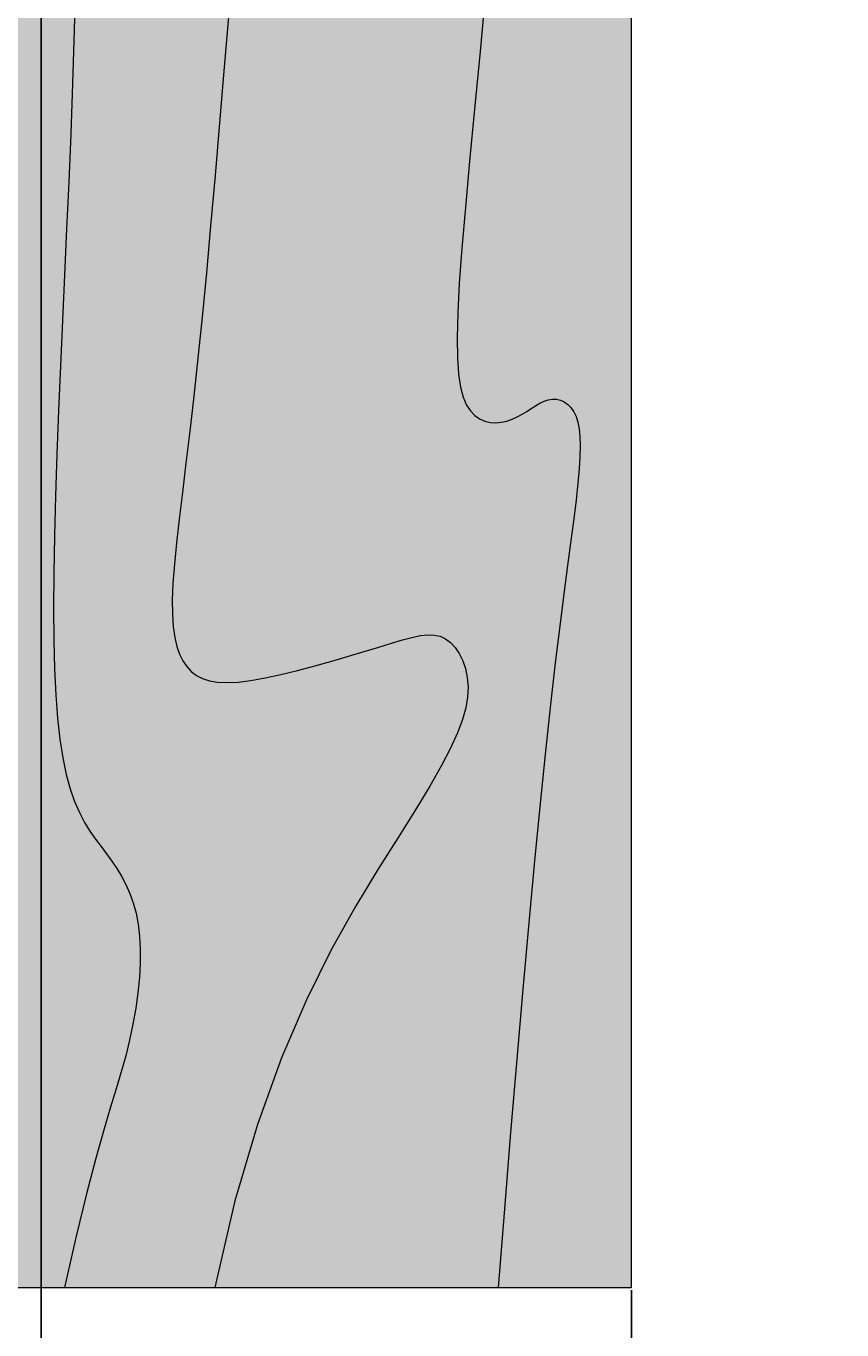
# Model space of a CAD drawing. Units: inches. Extents: x 2549 to 3108, y 1683 to 2362.
# Tile 25 of 30: x 2966 to 2985, y 2018 to 2049. Entities that reach past the tile are written whole.
import ezdxf

# ---------------------------------------------------------------- set-up
doc = ezdxf.new("R2010")
doc.units = ezdxf.units.IN
for name, color, linetype, lineweight in [('A-ANNO-DIMS', 2, 'Continuous', 18), ('A-FURN', 8, 'Continuous', 18), ('A-FURN-PATT', 9, 'Continuous', 13)]:
    doc.layers.add(name, color=color, linetype=linetype, lineweight=lineweight)
doc.layers.add('C-PKNG-VEHI-PATT', color=251, linetype='Continuous', lineweight=13, true_color=0x636466)
doc.layers.add('C-PVMT-PATT', color=9, linetype='Continuous', lineweight=13, true_color=0xc7c8ca)
doc.styles.get("Standard").update_dxf_attribs({"font": 'arial.ttf'})
doc.dimstyles.get("Standard").update_dxf_attribs({"dimtxt": 0.18, "dimasz": 0.18, "dimexe": 0.18, "dimexo": 0.0625, "dimgap": 0.09, "dimtad": 0, "dimtih": 1, "dimtoh": 1, "dimdec": 4, "dimzin": 0, "dimdsep": 46, "dimtxsty": 'Standard', "dimcen": 0.09, "dimadec": 0, "dimazin": 0, "dimtfac": 1, "dimtdec": 4, "dimtofl": 0, "dimtmove": 0, "dimatfit": 3, "dimfxl": 1, "dimtolj": 1, "dimtzin": 0, "dimarcsym": 0})

# ---------------------------------------------------------------- blocks, each defined once
blk = doc.blocks.new('Table - Rectangular Woodgrain 60 x 30 in.')
for p, q in [((60, 0), (0, 0)), ((60, -30), (60, 0))]:
    blk.add_line(p, q)
for points in [[(28.8172, -3.4958), (30.3437, -3.636), (31.7291, -3.7667), (32.9756, -3.8849), (34.0849, -3.9875), (35.059, -4.0714), (35.9, -4.1334), (36.6114, -4.1711), (37.2041, -4.1854), (37.6906, -4.1779), (38.0833, -4.15), (38.3948, -4.1034), (38.6375, -4.0396), (38.8239, -3.9602), (38.9666, -3.8667), (39.0764, -3.7608), (39.1573, -3.6448), (39.2116, -3.521), (39.2416, -3.3917), (39.2498, -3.2593), (39.2385, -3.1261), (39.21, -2.9944), (39.1666, -2.8667), (39.111, -2.7447), (39.0468, -2.6281), (38.978, -2.5163), (38.9083, -2.4083), (38.8418, -2.3035), (38.7823, -2.201), (38.7337, -2.1001), (38.7, -2), (38.6844, -1.9003), (38.6875, -1.8021), (38.7094, -1.707), (38.75, -1.6167), (38.8094, -1.5326), (38.8875, -1.4563), (38.9844, -1.3893), (39.1, -1.3333), (39.2351, -1.2896), (39.3937, -1.2583), (39.5804, -1.2396), (39.8, -1.2333), (40.057, -1.2396), (40.3562, -1.2583), (40.7023, -1.2896), (41.1, -1.3333), (41.5547, -1.3895), (42.0755, -1.4573), (42.6721, -1.5361), (43.3542, -1.625), (44.1316, -1.7233), (45.014, -1.8302), (46.0114, -1.9449), (47.1333, -2.0667), (48.3862, -2.1947), (49.7625, -2.3281), (51.2513, -2.4663), (52.8416, -2.6083), (54.5226, -2.7535), (56.2833, -2.9011), (58.1127, -3.0501), (60, -3.2)], [(29.3241, -9.6553), (30.7203, -9.7719), (32.0532, -9.8837), (33.3208, -9.9917), (34.5213, -10.0965), (35.6526, -10.199), (36.7128, -10.2999), (37.7, -10.4), (38.6129, -10.4996), (39.4531, -10.5969), (40.223, -10.6895), (40.925, -10.775), (41.5613, -10.8512), (42.1344, -10.9156), (42.6465, -10.966), (43.1, -11), (43.4976, -11.0158), (43.8437, -11.0136), (44.143, -10.9942), (44.4, -10.9583), (44.6195, -10.9069), (44.8062, -10.8406), (44.9648, -10.7603), (45.1, -10.6667), (45.2155, -10.5598), (45.3114, -10.4365), (45.3871, -10.2929), (45.4416, -10.125), (45.4743, -9.929), (45.4844, -9.7011), (45.4709, -9.4371), (45.4333, -9.1333), (45.3716, -8.7883), (45.2896, -8.4104), (45.1919, -8.0107), (45.0833, -7.6), (44.9685, -7.1893), (44.8521, -6.7896), (44.7388, -6.4117), (44.6333, -6.0667), (44.54, -5.7628), (44.4614, -5.4979), (44.4001, -5.2675), (44.3583, -5.0667), (44.3384, -4.8909), (44.3427, -4.7354), (44.3736, -4.5956), (44.4333, -4.4667), (44.5236, -4.3453), (44.6427, -4.2333), (44.7884, -4.1339), (44.9583, -4.05), (45.1501, -3.9849), (45.3614, -3.9417), (45.59, -3.9234), (45.8333, -3.9333), (46.0915, -3.9749), (46.3734, -4.0531), (46.6906, -4.1736), (47.0542, -4.3417), (47.4756, -4.5629), (47.9661, -4.8427), (48.5372, -5.1866), (49.2, -5.6), (49.9676, -6.0844), (50.8594, -6.625), (51.8965, -7.2031), (53.1, -7.8), (54.491, -8.3969), (56.0906, -8.975), (57.9199, -9.5156), (60, -10)], [(28.4531, -13.3281), (29.8256, -13.3663), (31.1083, -13.4083), (32.3191, -13.4535), (33.476, -13.501), (34.597, -13.5501), (35.7, -13.6), (36.7984, -13.6497), (37.8875, -13.6979), (38.9578, -13.743), (40, -13.7833), (41.0047, -13.8174), (41.9625, -13.8438), (42.864, -13.8607), (43.7, -13.8667), (44.4631, -13.8604), (45.1552, -13.8417), (45.7801, -13.8104), (46.3416, -13.7667), (46.8439, -13.7104), (47.2906, -13.6417), (47.6858, -13.5604), (48.0333, -13.4667), (48.3375, -13.3608), (48.6042, -13.2448), (48.8396, -13.121), (49.05, -12.9917), (49.2417, -12.8593), (49.4208, -12.7261), (49.5937, -12.5944), (49.7667, -12.4667), (49.9452, -12.3451), (50.1323, -12.2313), (50.3303, -12.1268), (50.5416, -12.0333), (50.7686, -11.9524), (51.0135, -11.8854), (51.2788, -11.8341), (51.5666, -11.8), (51.8785, -11.7843), (52.2116, -11.7865), (52.562, -11.8059), (52.926, -11.8417), (53.2998, -11.8931), (53.6795, -11.9594), (54.0614, -12.0397), (54.4416, -12.1333), (54.8223, -12.2401), (55.2293, -12.3625), (55.6942, -12.5037), (56.2489, -12.6667), (56.9251, -12.8547), (57.7545, -13.0708), (58.7689, -13.3182), (60, -13.6)]]:
    blk.add_lwpolyline(points)
blk = doc.blocks.new('*D23')
at = {"layer": 'A-ANNO-DIMS', "color": 0, "lineweight": -2, "transparency": 16777216}
for p, q in [((2950.093, 2018.552), (2950.093, 2009.435)), ((2980.093, 2018.552), (2980.093, 2009.435)), ((2950.273, 2009.615), (2964.875, 2009.615)), ((2979.913, 2009.615), (2965.312, 2009.615))]:
    blk.add_line(p, q, dxfattribs=at)
at = {"layer": 'A-ANNO-DIMS', "color": 0, "transparency": 16777216}
for points in [[(2950.273, 2009.645), (2950.273, 2009.585), (2950.093, 2009.615)], [(2979.913, 2009.645), (2979.913, 2009.585), (2980.093, 2009.615)]]:
    blk.add_solid(points, dxfattribs=at)
at = {"layer": 'Defpoints', "color": 0, "transparency": 16777216}
for p in [(2950.093, 2018.615), (2980.093, 2018.615), (2980.093, 2009.615)]:
    blk.add_point(p, dxfattribs=at)
at = {"layer": 'A-ANNO-DIMS', "color": 0, "transparency": 16777216, "insert": (2965.093, 2009.615), "char_height": 0.18, "attachment_point": 5}
blk.add_mtext('\\A1;30', dxfattribs=at)
blk = doc.blocks.new('*D46')
at = {"layer": 'A-ANNO-DIMS', "color": 0, "lineweight": -2, "transparency": 16777216}
for p, q in [((2812.643, 2140.461), (2812.643, 1683.444)), ((3034.643, 2134.461), (3034.643, 1683.444)), ((2812.823, 1683.624), (2923.353, 1683.624)), ((3034.463, 1683.624), (2923.932, 1683.624))]:
    blk.add_line(p, q, dxfattribs=at)
at = {"layer": 'A-ANNO-DIMS', "color": 0, "transparency": 16777216}
for points in [[(2812.823, 1683.654), (2812.823, 1683.594), (2812.643, 1683.624)], [(3034.463, 1683.654), (3034.463, 1683.594), (3034.643, 1683.624)]]:
    blk.add_solid(points, dxfattribs=at)
at = {"layer": 'Defpoints', "color": 0, "transparency": 16777216}
for p in [(2812.643, 2140.524), (3034.643, 2134.524), (3034.643, 1683.624)]:
    blk.add_point(p, dxfattribs=at)
at = {"layer": 'A-ANNO-DIMS', "color": 0, "transparency": 16777216, "insert": (2923.643, 1683.624), "char_height": 0.18, "attachment_point": 5}
blk.add_mtext('\\A1;222', dxfattribs=at)
blk = doc.blocks.new('*D57')
at = {"layer": 'A-ANNO-DIMS', "color": 0, "lineweight": -2, "transparency": 16777216}
for p, q in [((2965.935, 1936.586), (2965.935, 2362.323)), ((3034.643, 1936.586), (3034.643, 2362.323)), ((2966.115, 2362.143), (2999.912, 2362.143)), ((3034.463, 2362.143), (3000.666, 2362.143))]:
    blk.add_line(p, q, dxfattribs=at)
at = {"layer": 'A-ANNO-DIMS', "color": 0, "transparency": 16777216}
for points in [[(2966.115, 2362.173), (2966.115, 2362.113), (2965.935, 2362.143)], [(3034.463, 2362.173), (3034.463, 2362.113), (3034.643, 2362.143)]]:
    blk.add_solid(points, dxfattribs=at)
at = {"layer": 'Defpoints', "color": 0, "transparency": 16777216}
for p in [(3034.643, 2362.143), (2965.935, 1936.524), (3034.643, 1936.524)]:
    blk.add_point(p, dxfattribs=at)
at = {"layer": 'A-ANNO-DIMS', "color": 0, "transparency": 16777216, "insert": (3000.289, 2362.143), "char_height": 0.18, "attachment_point": 5}
blk.add_mtext('\\A1;68.71', dxfattribs=at)

msp = doc.modelspace()

# ---------------------------------------------------------------- hatches: boundary and pattern name
at = {"layer": 'A-FURN-PATT', "transparency": 33554684}
h = msp.add_hatch(color=256, dxfattribs=at)
h.dxf.hatch_style = 1
h.paths.add_polyline_path([(2951.6587, 2056.0021), (2951.6557, 2058.2435), (2951.6347, 2060.9396), (2951.5919, 2064.2076), (2951.5233, 2068.1646), (2951.425, 2072.9279), (2951.2931, 2078.6146), (2950.0931, 2078.6146), (2950.0931, 2018.6146), (2952.4931, 2018.6146), (2952.0883, 2021.7874), (2951.7676, 2024.5157), (2951.521, 2026.8517), (2951.3389, 2028.848), (2951.2115, 2030.5567), (2951.129, 2032.0303), (2951.0817, 2033.321), (2951.0598, 2034.4813), (2951.0547, 2035.5574), (2951.0634, 2036.5714), (2951.0838, 2037.5393), (2951.1139, 2038.4771), (2951.1519, 2039.4009), (2951.1957, 2040.3266), (2951.2434, 2041.2703), (2951.2931, 2042.248), (2951.343, 2043.2741), (2951.392, 2044.3568), (2951.4396, 2045.5028), (2951.4847, 2046.7188), (2951.5268, 2048.0113), (2951.565, 2049.387), (2951.5984, 2050.8526), (2951.6264, 2052.4146), (2951.6476, 2054.0982)])
h.paths.add_polyline_path([(2955.3325, 2057.2097), (2955.19, 2062.912), (2955.0427, 2069.9791), (2954.8931, 2078.6146), (2951.2931, 2078.6146), (2951.425, 2072.9279), (2951.5233, 2068.1646), (2951.5919, 2064.2076), (2951.6347, 2060.9396), (2951.6557, 2058.2435), (2951.6587, 2056.0021), (2951.6476, 2054.0982), (2951.6264, 2052.4146), (2951.5984, 2050.8526), (2951.565, 2049.387), (2951.5268, 2048.0113), (2951.4847, 2046.7188), (2951.4396, 2045.5028), (2951.392, 2044.3568), (2951.343, 2043.2741), (2951.2931, 2042.248), (2951.2434, 2041.2703), (2951.1957, 2040.3266), (2951.1519, 2039.4009), (2951.1139, 2038.4771), (2951.0838, 2037.5393), (2951.0634, 2036.5714), (2951.0547, 2035.5574), (2951.0598, 2034.4813), (2951.0817, 2033.321), (2951.129, 2032.0303), (2951.2115, 2030.5567), (2951.3389, 2028.848), (2951.521, 2026.8517), (2951.7676, 2024.5157), (2952.0883, 2021.7874), (2952.4931, 2018.6146), (2955.2931, 2018.6146), (2955.302, 2019.3711), (2955.3269, 2020.1382), (2955.3652, 2020.9125), (2955.4139, 2021.6907), (2955.4705, 2022.4692), (2955.5321, 2023.2447), (2955.5961, 2024.0137), (2955.6597, 2024.7729), (2955.7206, 2025.5211), (2955.778, 2026.2663), (2955.8314, 2027.0187), (2955.8806, 2027.7886), (2955.9251, 2028.5862), (2955.9644, 2029.4218), (2955.9984, 2030.3056), (2956.0264, 2031.2479), (2956.048, 2032.2589), (2956.0618, 2033.3479), (2956.0663, 2034.5245), (2956.0598, 2035.7979), (2956.0408, 2037.1776), (2956.0077, 2038.6729), (2955.959, 2040.2933), (2955.8931, 2042.0479), (2955.8091, 2043.9787), (2955.7087, 2046.2568), (2955.5943, 2049.0856), (2955.4681, 2052.6688)])
h.paths.add_polyline_path([(2958.1396, 2059.1978), (2957.992, 2064.2052), (2957.843, 2070.6048), (2957.6931, 2078.6146), (2954.8931, 2078.6146), (2955.0427, 2069.9791), (2955.19, 2062.912), (2955.3325, 2057.2097), (2955.4681, 2052.6688), (2955.5943, 2049.0856), (2955.7087, 2046.2568), (2955.8091, 2043.9787), (2955.8931, 2042.0479), (2955.959, 2040.2933), (2956.0077, 2038.6729), (2956.0408, 2037.1776), (2956.0598, 2035.7979), (2956.0663, 2034.5245), (2956.0618, 2033.3479), (2956.048, 2032.2589), (2956.0264, 2031.2479), (2955.9984, 2030.3056), (2955.9644, 2029.4218), (2955.9251, 2028.5862), (2955.8806, 2027.7886), (2955.8314, 2027.0187), (2955.778, 2026.2663), (2955.7206, 2025.5211), (2955.6597, 2024.7729), (2955.5961, 2024.0137), (2955.5321, 2023.2447), (2955.4705, 2022.4692), (2955.4139, 2021.6907), (2955.3652, 2020.9125), (2955.3269, 2020.1382), (2955.302, 2019.3711), (2955.2931, 2018.6146), (2958.4931, 2018.6146), (2958.3701, 2019.0734), (2958.2967, 2019.5472), (2958.2663, 2020.0323), (2958.2723, 2020.525), (2958.3079, 2021.0217), (2958.3665, 2021.5185), (2958.4416, 2022.0118), (2958.5264, 2022.4979), (2958.6154, 2022.9752), (2958.7072, 2023.45), (2958.8012, 2023.9312), (2958.8973, 2024.4271), (2958.9948, 2024.9465), (2959.0936, 2025.498), (2959.1932, 2026.09), (2959.2931, 2026.7313), (2959.3927, 2027.4274), (2959.49, 2028.1717), (2959.5825, 2028.9546), (2959.6681, 2029.7667), (2959.7443, 2030.5983), (2959.8087, 2031.4399), (2959.8591, 2032.2818), (2959.8931, 2033.1146), (2959.909, 2033.931), (2959.9077, 2034.7334), (2959.8907, 2035.5263), (2959.8598, 2036.3146), (2959.8163, 2037.1029), (2959.7618, 2037.8959), (2959.698, 2038.6982), (2959.6264, 2039.5146), (2959.5483, 2040.3504), (2959.4639, 2041.2131), (2959.3733, 2042.1109), (2959.2764, 2043.0521), (2959.1733, 2044.0449), (2959.0639, 2045.0974), (2958.9483, 2046.2179), (2958.8264, 2047.4146), (2958.6984, 2048.7306), (2958.565, 2050.349), (2958.4268, 2052.4877), (2958.2848, 2055.3646)])
h.paths.add_polyline_path([(2963.0634, 2055.4818), (2962.9958, 2058.2679), (2962.8973, 2061.4021), (2962.7628, 2064.9441), (2962.5874, 2068.9537), (2962.3658, 2073.4906), (2962.0931, 2078.6146), (2957.6931, 2078.6146), (2957.843, 2070.6048), (2957.992, 2064.2052), (2958.1396, 2059.1978), (2958.2848, 2055.3646), (2958.4268, 2052.4877), (2958.565, 2050.349), (2958.6984, 2048.7306), (2958.8264, 2047.4146), (2958.9483, 2046.2179), (2959.0639, 2045.0974), (2959.1733, 2044.0449), (2959.2764, 2043.0521), (2959.3733, 2042.1109), (2959.4639, 2041.2131), (2959.5483, 2040.3504), (2959.6264, 2039.5146), (2959.698, 2038.6982), (2959.7618, 2037.8959), (2959.8163, 2037.1029), (2959.8598, 2036.3146), (2959.8907, 2035.5263), (2959.9077, 2034.7334), (2959.909, 2033.931), (2959.8931, 2033.1146), (2959.8591, 2032.2818), (2959.8087, 2031.4399), (2959.7443, 2030.5983), (2959.6681, 2029.7667), (2959.5825, 2028.9546), (2959.49, 2028.1717), (2959.3927, 2027.4274), (2959.2931, 2026.7313), (2959.1932, 2026.09), (2959.0936, 2025.498), (2958.9948, 2024.9465), (2958.8973, 2024.4271), (2958.8012, 2023.9312), (2958.7072, 2023.45), (2958.6154, 2022.9752), (2958.5264, 2022.4979), (2958.4416, 2022.0118), (2958.3665, 2021.5185), (2958.3079, 2021.0217), (2958.2723, 2020.525), (2958.2663, 2020.0323), (2958.2967, 2019.5472), (2958.3701, 2019.0734), (2958.4931, 2018.6146), (2962.8931, 2018.6146), (2962.8935, 2018.8741), (2962.9256, 2019.0114), (2962.9493, 2019.1068), (2962.9824, 2019.2467), (2963.0264, 2019.448), (2963.082, 2019.7222), (2963.1462, 2020.0607), (2963.2151, 2020.4496), (2963.2847, 2020.875), (2963.3513, 2021.3231), (2963.4108, 2021.78), (2963.4594, 2022.2318), (2963.4931, 2022.6646), (2963.509, 2023.0681), (2963.5077, 2023.4453), (2963.4907, 2023.8031), (2963.4597, 2024.148), (2963.4163, 2024.4866), (2963.3618, 2024.8256), (2963.298, 2025.1716), (2963.2264, 2025.5313), (2963.1488, 2025.9112), (2963.0681, 2026.3175), (2962.9874, 2026.7562), (2962.9098, 2027.2334), (2962.8384, 2027.7551), (2962.7764, 2028.3274), (2962.7269, 2028.9563), (2962.6931, 2029.6479), (2962.6771, 2030.4072), (2962.6775, 2031.2344), (2962.6919, 2032.1288), (2962.7181, 2033.0896), (2962.7536, 2034.116), (2962.7962, 2035.2073), (2962.8435, 2036.3627), (2962.8931, 2037.5813), (2962.9428, 2038.8647), (2962.9905, 2040.224), (2963.0343, 2041.6723), (2963.0723, 2043.2229), (2963.1024, 2044.8892), (2963.1228, 2046.6844), (2963.1314, 2048.6218), (2963.1264, 2050.7146), (2963.1053, 2052.9839)])
h.paths.add_polyline_path([(2967.0608, 2068.9933), (2967.1609, 2073.4299), (2967.2931, 2078.6146), (2962.0931, 2078.6146), (2962.3658, 2073.4906), (2962.5874, 2068.9537), (2962.7628, 2064.9441), (2962.8973, 2061.4021), (2962.9958, 2058.2679), (2963.0634, 2055.4818), (2963.1053, 2052.9839), (2963.1264, 2050.7146), (2963.1314, 2048.6218), (2963.1228, 2046.6844), (2963.1024, 2044.8892), (2963.0723, 2043.2229), (2963.0343, 2041.6723), (2962.9905, 2040.224), (2962.9428, 2038.8647), (2962.8931, 2037.5813), (2962.8435, 2036.3627), (2962.7962, 2035.2073), (2962.7536, 2034.116), (2962.7181, 2033.0896), (2962.6919, 2032.1288), (2962.6775, 2031.2344), (2962.6771, 2030.4072), (2962.6931, 2029.6479), (2962.7269, 2028.9563), (2962.7764, 2028.3274), (2962.8384, 2027.7551), (2962.9098, 2027.2334), (2962.9874, 2026.7562), (2963.0681, 2026.3175), (2963.1488, 2025.9112), (2963.2264, 2025.5313), (2963.298, 2025.1716), (2963.3618, 2024.8256), (2963.4163, 2024.4866), (2963.4597, 2024.148), (2963.4907, 2023.8031), (2963.5077, 2023.4453), (2963.509, 2023.0681), (2963.4931, 2022.6646), (2963.4594, 2022.2318), (2963.4108, 2021.78), (2963.3513, 2021.3231), (2963.2847, 2020.875), (2963.2151, 2020.4496), (2963.1462, 2020.0607), (2963.082, 2019.7222), (2963.0264, 2019.448), (2962.9824, 2019.2467), (2962.9493, 2019.1068), (2962.9256, 2019.0114), (2962.9098, 2018.9438), (2962.9001, 2018.8871), (2962.8952, 2018.8245), (2962.8933, 2018.7393), (2962.8931, 2018.6146), (2966.4931, 2018.6146), (2966.7749, 2019.8457), (2967.0223, 2020.8601), (2967.2384, 2021.6895), (2967.4264, 2022.3657), (2967.5894, 2022.9204), (2967.7306, 2023.3853), (2967.853, 2023.7923), (2967.9598, 2024.173), (2968.0534, 2024.5532), (2968.1337, 2024.9351), (2968.2, 2025.3148), (2968.2514, 2025.6886), (2968.2872, 2026.0526), (2968.3066, 2026.403), (2968.3088, 2026.7361), (2968.2931, 2027.048), (2968.259, 2027.3358), (2968.2077, 2027.6011), (2968.1407, 2027.846), (2968.0598, 2028.073), (2967.9663, 2028.2843), (2967.8618, 2028.4823), (2967.748, 2028.6694), (2967.6264, 2028.8479), (2967.4987, 2029.0209), (2967.367, 2029.1938), (2967.2338, 2029.3729), (2967.1014, 2029.5646), (2966.9721, 2029.775), (2966.8483, 2030.0104), (2966.7323, 2030.2771), (2966.6264, 2030.5813), (2966.5327, 2030.9288), (2966.4514, 2031.324), (2966.3827, 2031.7707), (2966.3264, 2032.273), (2966.2827, 2032.8345), (2966.2514, 2033.4594), (2966.2327, 2034.1515), (2966.2264, 2034.9146), (2966.2324, 2035.7506), (2966.2493, 2036.6521), (2966.2757, 2037.6099), (2966.3098, 2038.6146), (2966.3501, 2039.6568), (2966.3952, 2040.7271), (2966.4434, 2041.8162), (2966.4931, 2042.9146), (2966.543, 2044.0176), (2966.5921, 2045.1386), (2966.6396, 2046.2955), (2966.6848, 2047.5063), (2966.7268, 2048.789), (2966.765, 2050.1615), (2966.7984, 2051.6418), (2966.8264, 2053.248), (2966.8492, 2055.0092), (2966.8712, 2057.0006), (2966.8979, 2059.3083), (2966.9348, 2062.0188), (2966.9872, 2065.2183)])
h.paths.add_polyline_path([(2971.0073, 2072.0387), (2970.8931, 2078.6146), (2967.2931, 2078.6146), (2967.1609, 2073.4299), (2967.0608, 2068.9933), (2966.9872, 2065.2183), (2966.9348, 2062.0188), (2966.8979, 2059.3083), (2966.8712, 2057.0006), (2966.8492, 2055.0092), (2966.8264, 2053.248), (2966.7984, 2051.6418), (2966.765, 2050.1615), (2966.7268, 2048.789), (2966.6848, 2047.5063), (2966.6396, 2046.2955), (2966.5921, 2045.1386), (2966.543, 2044.0176), (2966.4931, 2042.9146), (2966.4434, 2041.8162), (2966.3952, 2040.7271), (2966.3501, 2039.6568), (2966.3098, 2038.6146), (2966.2757, 2037.6099), (2966.2493, 2036.6521), (2966.2324, 2035.7506), (2966.2264, 2034.9146), (2966.2327, 2034.1515), (2966.2514, 2033.4594), (2966.2827, 2032.8345), (2966.3264, 2032.273), (2966.3827, 2031.7707), (2966.4514, 2031.324), (2966.5327, 2030.9288), (2966.6264, 2030.5813), (2966.7323, 2030.2771), (2966.8483, 2030.0104), (2966.9721, 2029.775), (2967.1014, 2029.5646), (2967.2338, 2029.3729), (2967.367, 2029.1938), (2967.4987, 2029.0209), (2967.6264, 2028.8479), (2967.748, 2028.6694), (2967.8618, 2028.4823), (2967.9663, 2028.2843), (2968.0598, 2028.073), (2968.1407, 2027.846), (2968.2077, 2027.6011), (2968.259, 2027.3358), (2968.2931, 2027.048), (2968.3088, 2026.7361), (2968.3066, 2026.403), (2968.2872, 2026.0526), (2968.2514, 2025.6886), (2968.2, 2025.3148), (2968.1337, 2024.9351), (2968.0534, 2024.5532), (2967.9598, 2024.173), (2967.853, 2023.7923), (2967.7306, 2023.3853), (2967.5894, 2022.9204), (2967.4264, 2022.3657), (2967.2384, 2021.6895), (2967.0223, 2020.8601), (2966.7749, 2019.8457), (2966.4931, 2018.6146), (2970.0931, 2018.6146), (2970.5775, 2020.6947), (2971.1181, 2022.524), (2971.6962, 2024.1236), (2972.2931, 2025.5146), (2972.89, 2026.7181), (2973.4681, 2027.7552), (2974.0087, 2028.647), (2974.4931, 2029.4146), (2974.9065, 2030.0774), (2975.2504, 2030.6485), (2975.5302, 2031.139), (2975.7514, 2031.5604), (2975.9195, 2031.924), (2976.04, 2032.2412), (2976.1182, 2032.5231), (2976.1598, 2032.7813), (2976.1697, 2033.0246), (2976.1514, 2033.2532), (2976.1082, 2033.4645), (2976.0431, 2033.6563), (2975.9592, 2033.8262), (2975.8598, 2033.9719), (2975.7478, 2034.091), (2975.6264, 2034.1813), (2975.4975, 2034.241), (2975.3577, 2034.2719), (2975.2022, 2034.2762), (2975.0264, 2034.2563), (2974.8256, 2034.2145), (2974.5952, 2034.1532), (2974.3303, 2034.0746), (2974.0264, 2033.9813), (2973.6814, 2033.8758), (2973.3035, 2033.7625), (2972.9038, 2033.6461), (2972.4931, 2033.5313), (2972.0824, 2033.4227), (2971.6827, 2033.325), (2971.3048, 2033.243), (2970.9598, 2033.1813), (2970.656, 2033.1437), (2970.392, 2033.1302), (2970.1641, 2033.1403), (2969.9681, 2033.173), (2969.8002, 2033.2275), (2969.6566, 2033.3032), (2969.5333, 2033.3991), (2969.4264, 2033.5146), (2969.3328, 2033.6498), (2969.2525, 2033.8084), (2969.1862, 2033.9951), (2969.1348, 2034.2146), (2969.0989, 2034.4716), (2969.0795, 2034.7709), (2969.0773, 2035.117), (2969.0931, 2035.5146), (2969.1271, 2035.9681), (2969.1775, 2036.4802), (2969.2419, 2037.0533), (2969.3181, 2037.6896), (2969.4036, 2038.3916), (2969.4962, 2039.1615), (2969.5935, 2040.0017), (2969.6931, 2040.9146), (2969.7932, 2041.9018), (2969.8941, 2042.962), (2969.9966, 2044.0933), (2970.1014, 2045.2938), (2970.2094, 2046.5614), (2970.3212, 2047.8943), (2970.4378, 2049.2905), (2970.5598, 2050.748), (2970.6862, 2052.2926), (2970.8087, 2054.0615), (2970.9172, 2056.2194), (2971.0014, 2058.9313), (2971.0513, 2062.3619), (2971.0566, 2066.6761)])
h.paths.add_polyline_path([(2977.5454, 2065.9056), (2977.6243, 2069.5844), (2977.6751, 2073.7991), (2977.6931, 2078.6146), (2970.8931, 2078.6146), (2971.0073, 2072.0387), (2971.0566, 2066.6761), (2971.0513, 2062.3619), (2971.0014, 2058.9313), (2970.9172, 2056.2194), (2970.8087, 2054.0615), (2970.6862, 2052.2926), (2970.5598, 2050.748), (2970.4378, 2049.2905), (2970.3212, 2047.8943), (2970.2094, 2046.5614), (2970.1014, 2045.2938), (2969.9966, 2044.0933), (2969.8941, 2042.962), (2969.7932, 2041.9018), (2969.6931, 2040.9146), (2969.5935, 2040.0017), (2969.4962, 2039.1615), (2969.4036, 2038.3916), (2969.3181, 2037.6896), (2969.2419, 2037.0533), (2969.1775, 2036.4802), (2969.1271, 2035.9681), (2969.0931, 2035.5146), (2969.0773, 2035.117), (2969.0795, 2034.7709), (2969.0989, 2034.4716), (2969.1348, 2034.2146), (2969.1862, 2033.9951), (2969.2525, 2033.8084), (2969.3328, 2033.6498), (2969.4264, 2033.5146), (2969.5333, 2033.3991), (2969.6566, 2033.3032), (2969.8002, 2033.2275), (2969.9681, 2033.173), (2970.1641, 2033.1403), (2970.392, 2033.1302), (2970.656, 2033.1437), (2970.9598, 2033.1813), (2971.3048, 2033.243), (2971.6827, 2033.325), (2972.0824, 2033.4227), (2972.4931, 2033.5313), (2972.9038, 2033.6461), (2973.3035, 2033.7625), (2973.6814, 2033.8758), (2974.0264, 2033.9813), (2974.3303, 2034.0746), (2974.5952, 2034.1532), (2974.8256, 2034.2145), (2975.1314, 2034.2781), (2975.4354, 2034.2697), (2975.6264, 2034.1813), (2975.7478, 2034.091), (2975.8598, 2033.9719), (2975.9592, 2033.8262), (2976.0431, 2033.6563), (2976.1082, 2033.4645), (2976.1514, 2033.2532), (2976.1697, 2033.0246), (2976.1598, 2032.7813), (2976.1182, 2032.5231), (2976.04, 2032.2412), (2975.9195, 2031.924), (2975.7514, 2031.5604), (2975.5302, 2031.139), (2975.2504, 2030.6485), (2974.9065, 2030.0774), (2974.4931, 2029.4146), (2974.0087, 2028.647), (2973.4681, 2027.7552), (2972.89, 2026.7181), (2972.2931, 2025.5146), (2971.6962, 2024.1236), (2971.1181, 2022.524), (2970.5775, 2020.6947), (2970.0931, 2018.6146), (2976.8931, 2018.6146), (2977.043, 2020.5019), (2977.192, 2022.3313), (2977.3396, 2024.092), (2977.4848, 2025.773), (2977.6268, 2027.3633), (2977.765, 2028.8521), (2977.8984, 2030.2284), (2978.0264, 2031.4813), (2978.1482, 2032.6032), (2978.2629, 2033.6006), (2978.3698, 2034.483), (2978.4681, 2035.2604), (2978.557, 2035.9425), (2978.6358, 2036.5391), (2978.7036, 2037.0599), (2978.7598, 2037.5146), (2978.8035, 2037.9123), (2978.8348, 2038.2584), (2978.8535, 2038.5576), (2978.8598, 2038.8146), (2978.8535, 2039.0342), (2978.8348, 2039.2209), (2978.8035, 2039.3795), (2978.7598, 2039.5146), (2978.7038, 2039.6302), (2978.6368, 2039.7271), (2978.5605, 2039.8052), (2978.4764, 2039.8646), (2978.3861, 2039.9052), (2978.291, 2039.9271), (2978.1928, 2039.9302), (2978.0931, 2039.9146), (2977.993, 2039.8809), (2977.8921, 2039.8323), (2977.7896, 2039.7728), (2977.6848, 2039.7063), (2977.5003, 2039.5872), (2977.2813, 2039.4666), (2977.0307, 2039.3815), (2976.7627, 2039.3587), (2976.5032, 2039.4189), (2976.3323, 2039.5382), (2976.2264, 2039.648), (2976.1329, 2039.7907), (2976.0535, 2039.9771), (2975.9897, 2040.2198), (2975.9431, 2040.5313), (2975.9152, 2040.924), (2975.9077, 2041.4105), (2975.922, 2042.0032), (2975.9597, 2042.7146), (2976.0217, 2043.5556), (2976.1056, 2044.5297), (2976.2082, 2045.639), (2976.3264, 2046.8855), (2976.4571, 2048.2709), (2976.5973, 2049.7974), (2976.7436, 2051.4669), (2976.8931, 2053.2813), (2977.0423, 2055.253), (2977.1868, 2057.4365), (2977.322, 2059.8965), (2977.4431, 2062.6979)])
h.paths.add_polyline_path([(2980.0931, 2078.6146), (2977.6931, 2078.6146), (2977.6751, 2073.7991), (2977.6243, 2069.5844), (2977.5454, 2065.9056), (2977.4431, 2062.6979), (2977.322, 2059.8965), (2977.1868, 2057.4365), (2977.0423, 2055.253), (2976.8931, 2053.2813), (2976.7436, 2051.4669), (2976.5973, 2049.7974), (2976.4571, 2048.2709), (2976.3264, 2046.8855), (2976.2082, 2045.639), (2976.1056, 2044.5297), (2976.0217, 2043.5556), (2975.9597, 2042.7146), (2975.922, 2042.0032), (2975.9077, 2041.4105), (2975.9152, 2040.924), (2975.9431, 2040.5313), (2975.9897, 2040.2198), (2976.0535, 2039.9771), (2976.1329, 2039.7907), (2976.2264, 2039.648), (2976.3323, 2039.5382), (2976.4483, 2039.4573), (2976.5721, 2039.403), (2976.7014, 2039.373), (2976.8338, 2039.3648), (2976.967, 2039.3761), (2977.0987, 2039.4046), (2977.2264, 2039.448), (2977.3484, 2039.5036), (2977.465, 2039.5678), (2977.5768, 2039.6366), (2977.7721, 2039.7626), (2977.9521, 2039.8671), (2978.144, 2039.9317), (2978.3409, 2039.9255), (2978.5228, 2039.8437), (2978.6765, 2039.6863), (2978.7598, 2039.5146), (2978.8035, 2039.3795), (2978.8348, 2039.2209), (2978.8535, 2039.0342), (2978.8598, 2038.8146), (2978.8535, 2038.5576), (2978.8348, 2038.2584), (2978.8035, 2037.9123), (2978.7598, 2037.5146), (2978.7036, 2037.0599), (2978.6358, 2036.5391), (2978.557, 2035.9425), (2978.4681, 2035.2604), (2978.3698, 2034.483), (2978.2629, 2033.6006), (2978.1482, 2032.6032), (2978.0264, 2031.4813), (2977.8984, 2030.2284), (2977.765, 2028.8521), (2977.6268, 2027.3633), (2977.4848, 2025.773), (2977.3396, 2024.092), (2977.192, 2022.3313), (2977.043, 2020.5019), (2976.8931, 2018.6146), (2980.0931, 2018.6146)])
at = {"layer": 'C-PKNG-VEHI-PATT'}
h = msp.add_hatch(color=256, dxfattribs=at)
h.dxf.hatch_style = 1
edge = h.paths.add_edge_path()
edge.add_ellipse((2935.7258, 1791.964), major_axis=(-50.66, 0), ratio=0.8423039, start_angle=248.16505, end_angle=265.72258)
edge.add_line((2938.911, 1834.5507), (2925.8653, 1834.5507))
edge.add_ellipse((2929.0505, 1791.964), major_axis=(50.66, 0), ratio=0.8423039, start_angle=94.27742, end_angle=111.83495)
edge.add_line((2912.8508, 1832.3947), (2914.2044, 1822.2495))
edge.add_ellipse((2930.6538, 1783.1023), major_axis=(-49.3014, 0), ratio=0.8423039, start_angle=-85.12993, end_angle=-67.20809, ccw=False)
edge.add_line((2927.1247, 1824.5225), (2937.6516, 1824.5225))
edge.add_ellipse((2934.1225, 1783.1023), major_axis=(49.3014, 0), ratio=0.8423039, start_angle=67.20809, end_angle=85.12993, ccw=False)
edge.add_line((2950.5719, 1822.2495), (2951.9255, 1832.3947))
edge = h.paths.add_edge_path()
edge.add_ellipse((2903.4793, 1857.3351), major_axis=(-34.7979, 0), ratio=0.8423039, start_angle=180, end_angle=209.43857)
edge.add_ellipse((2961.297, 1857.3351), major_axis=(34.7979, 0), ratio=0.8423039, start_angle=150.56143, end_angle=180)
edge.add_line((2926.4991, 1857.3351), (2926.4991, 1843.7609))
edge.add_ellipse((2924.1251, 1844.3143), major_axis=(-0.2209, 3.9278), ratio=0.6038336, start_angle=89.00201, end_angle=253.65741, ccw=False)
edge.add_line((2921.7512, 1844.2222), (2921.7512, 1853.3975))
edge.add_line((2921.7512, 1853.3975), (2925.269, 1855.8484))
edge.add_ellipse((2925.4782, 1855.4931), major_axis=(0.4584, 0), ratio=0.8423039, start_angle=90, end_angle=134.48021, ccw=False)
edge.add_line((2925.4782, 1855.8792), (2926.4991, 1855.8792))
edge.add_line((2926.4991, 1855.8792), (2926.4991, 1857.3351))
edge.add_ellipse((2961.297, 1857.3351), major_axis=(34.7979, 0), ratio=0.8423039, start_angle=150.56143, end_angle=180, ccw=False)
edge.add_line((2932.3882, 1873.6501), (2932.3882, 1875.7801))
edge.add_ellipse((2932.3882, 1875.3939), major_axis=(0.4584, 0), ratio=0.8423039, start_angle=90, end_angle=127.93313)
edge.add_line((2932.1366, 1875.7167), (2928.5915, 1873.7564))
edge.add_ellipse((2899.9271, 2002.4692), major_axis=(155.4756, 0), ratio=0.84230387, start_angle=-80.743434, end_angle=-77.445067, ccw=False)
edge.add_ellipse((2949.4402, 1715.2151), major_axis=(-189.1422, 0), ratio=0.84230387, start_angle=-79.790461, end_angle=-77.555373)
edge.add_ellipse((3300.3614, 1852.5642), major_axis=(-386.1662, 0), ratio=0.84230387, start_angle=-2.863715, end_angle=2.198541)
edge.add_ellipse((2929.0505, 1792.5159), major_axis=(-55.6192, 0), ratio=0.8423039, start_angle=-85.91759, end_angle=-72.28005, ccw=False)
edge.add_line((2925.7129, 1839.2798), (2939.0634, 1839.2798))
edge.add_ellipse((2935.7258, 1792.5159), major_axis=(55.6192, 0), ratio=0.8423039, start_angle=72.28005, end_angle=85.91759, ccw=False)
edge.add_ellipse((2564.4149, 1852.5642), major_axis=(-386.1662, 0), ratio=0.84230387, start_angle=177.801459, end_angle=182.863715)
edge.add_ellipse((2915.3361, 1715.2151), major_axis=(189.1422, 0), ratio=0.84230387, start_angle=77.555373, end_angle=79.790461)
edge.add_ellipse((2964.8492, 2002.4692), major_axis=(-155.4756, 0), ratio=0.84230387, start_angle=77.445067, end_angle=80.743434, ccw=False)
edge.add_line((2936.1848, 1873.7564), (2932.6397, 1875.7167))
edge.add_ellipse((2932.3882, 1875.3939), major_axis=(0.4584, 0), ratio=0.8423039, start_angle=52.06687, end_angle=90)
edge.add_line((2932.3882, 1875.7801), (2932.3882, 1873.6501))
edge.add_ellipse((2903.4793, 1857.3351), major_axis=(-34.7979, 0), ratio=0.8423039, start_angle=180, end_angle=209.43857, ccw=False)
edge.add_line((2938.2772, 1857.3351), (2938.2772, 1855.8792))
edge.add_line((2938.2772, 1855.8792), (2939.4059, 1855.8792))
edge.add_ellipse((2939.2981, 1855.4931), major_axis=(-0.4584, 0), ratio=0.8423039, start_angle=225.51979, end_angle=270, ccw=False)
edge.add_line((2939.5903, 1855.7906), (2943.0251, 1853.3975))
edge.add_line((2943.0251, 1853.3975), (2943.0251, 1844.2222))
edge.add_ellipse((2940.6512, 1844.3143), major_axis=(0.2209, 3.9278), ratio=0.6038336, start_angle=106.34259, end_angle=270.99799, ccw=False)
edge.add_line((2938.2772, 1843.7609), (2938.2772, 1857.3351))
edge = h.paths.add_edge_path()
edge.add_ellipse((2932.3882, 1865.1973), major_axis=(91.081, 0), ratio=0.8423039, start_angle=256.401865, end_angle=283.598135, ccw=False)
edge.add_line((2914.2044, 1790.0239), (2914.2044, 1778.3622))
edge.add_ellipse((2932.3882, 1853.5356), major_axis=(91.081, 0), ratio=0.8423039, start_angle=256.401865, end_angle=283.598135)
edge.add_line((2950.5719, 1778.3622), (2950.5719, 1790.0239))
edge = h.paths.add_edge_path()
edge.add_ellipse((2948.7383, 1772.3145), major_axis=(1.8336, 0), ratio=0.8423039, start_angle=0, end_angle=90)
edge.add_line((2948.7383, 1773.859), (2916.038, 1773.859))
edge.add_ellipse((2916.038, 1772.3145), major_axis=(1.8336, 0), ratio=0.8423039, start_angle=90, end_angle=180)
edge.add_line((2914.2044, 1772.3145), (2914.2044, 1760.2558))
edge.add_line((2914.2044, 1760.2558), (2950.5719, 1760.2558))
edge.add_line((2950.5719, 1760.2558), (2950.5719, 1772.3145))
h.paths.add_polyline_path([(2748.8496, 2101.6383), (2798.148, 2101.6383), (2798.148, 2111.4248), (2748.8496, 2111.4248)], flags=9)
h.paths.add_polyline_path([(2685.2081, 2101.489), (2719.3253, 2101.489), (2719.3253, 2111.2819), (2685.2081, 2111.2819)], flags=9)
h.paths.add_polyline_path([(2814.6852, 1907.1328), (2847.8384, 1907.1328), (2847.8384, 1916.9258), (2814.6852, 1916.9258)], flags=9)
h.paths.add_polyline_path([(2814.3906, 1835.5864), (2848.0172, 1835.5864), (2848.0172, 1845.3794), (2814.3906, 1845.3794)], flags=9)
h.paths.add_polyline_path([(2800.5245, 1759.1674), (2853.7435, 1759.1674), (2853.7435, 1768.954), (2800.5245, 1768.954)], flags=9)
h.paths.add_polyline_path([(2972.4611, 1807.3305), (3015.3943, 1807.3305), (3015.3943, 1817.117), (2972.4611, 1817.117)], flags=9)
h.paths.add_polyline_path([(2902.3327, 1888.6731), (2937.9131, 1888.6731), (2937.9131, 1898.4661), (2902.3327, 1898.4661)], flags=9)
h.paths.add_polyline_path([(2712.1779, 1878.9039), (2754.1257, 1878.9039), (2754.1257, 1888.6904), (2712.1779, 1888.6904)], flags=9)
h.paths.add_polyline_path([(2614.0056, 2012.812), (2650.0251, 2012.812), (2650.0251, 2022.4371), (2614.0056, 2022.4371)], flags=9)
h.paths.add_polyline_path([(2713.3129, 2003.1645), (2747.4237, 2003.1645), (2747.4237, 2012.951), (2713.3129, 2012.951)], flags=9)
h.paths.add_polyline_path([(2950.1379, 2001.6934), (2982.2992, 2001.6934), (2982.2992, 2011.48), (2950.1379, 2011.48)], flags=9)
h.paths.add_polyline_path([(2940.864, 2238.5537), (2997.5066, 2238.5537), (2997.5066, 2248.3466), (2940.864, 2248.3466)], flags=9)
h.paths.add_polyline_path([(2821.5457, 2202.8348), (2855.663, 2202.8348), (2855.663, 2212.6278), (2821.5457, 2212.6278)], flags=9)
h.paths.add_polyline_path([(2661.8026, 2238.6249), (2718.4451, 2238.6249), (2718.4451, 2248.4179), (2661.8026, 2248.4179)], flags=9)
at = {"layer": 'C-PVMT-PATT'}
h = msp.add_hatch(color=256, dxfattribs=at)
h.dxf.hatch_style = 1
h.paths.add_polyline_path([(3067.6427, 2305.5237), (2605.6427, 2305.5237), (2605.6427, 2074.5237), (2629.6427, 2074.5237), (2629.6427, 2281.5237), (3043.6427, 2281.5237), (3043.6427, 1885.5237), (3043.6427, 1872.8745), (3031.1672, 1872.8745), (3031.1672, 1862.5731), (2995.8054, 1862.5731), (2995.8054, 1872.8745), (2983.1752, 1872.8745), (2983.1752, 1885.5237), (2881.6427, 1885.5237), (2881.6427, 1795.5237), (2751.0977, 1795.5237), (2751.0977, 1761.5237), (2786.1577, 1761.5237), (2786.1577, 1723.5237), (2881.84, 1723.5237), (2881.84, 1714.5237), (3067.6427, 1714.5237), (3067.6427, 1723.5237)])
edge = h.paths.add_edge_path(flags=16)
edge.add_ellipse((2949.4402, 1710.9683), major_axis=(-194.1014, 0), ratio=0.84230387, start_angle=-77.874034, end_angle=-76.219471, ccw=False)
edge.add_ellipse((2949.4402, 1715.2151), major_axis=(-189.1422, 0), ratio=0.84230387, start_angle=-79.790461, end_angle=-77.555373, ccw=False)
edge.add_ellipse((2899.9271, 2002.4692), major_axis=(155.4756, 0), ratio=0.84230387, start_angle=-80.743434, end_angle=-77.445067)
edge.add_line((2928.5915, 1873.7564), (2932.3882, 1875.8558))
edge.add_line((2932.3882, 1875.8558), (2936.1848, 1873.7564))
edge.add_ellipse((2964.8492, 2002.4692), major_axis=(-155.4756, 0), ratio=0.84230387, start_angle=77.445067, end_angle=80.743434)
edge.add_ellipse((2915.3361, 1715.2151), major_axis=(189.1422, 0), ratio=0.84230387, start_angle=77.555373, end_angle=79.790461, ccw=False)
edge.add_ellipse((2915.3361, 1710.9683), major_axis=(-194.1014, 0), ratio=0.84230387, start_angle=256.219471, end_angle=257.874034, ccw=False)
edge.add_ellipse((2628.2871, 1850.2612), major_axis=(-327.2532, 0), ratio=0.84230387, start_angle=182.17995, end_angle=183.650428, ccw=False)
edge.add_ellipse((2955.5637, 1861.9334), major_axis=(-0.9168, 0), ratio=0.8423039, start_angle=180, end_angle=270, ccw=False)
edge.add_line((2956.4805, 1862.3857), (2956.4805, 1846.4866))
edge.add_ellipse((2955.5637, 1846.939), major_axis=(-0.9168, 0), ratio=0.8423039, start_angle=90, end_angle=180, ccw=False)
edge.add_ellipse((-3607.0606, 1835.832), major_axis=(-6562.6242, 0), ratio=0.84230387, start_angle=179.61613322, end_angle=180.09022909, ccw=False)
edge.add_ellipse((2955.5637, 1791.0926), major_axis=(0.9168, 0), ratio=0.8423039, start_angle=0, end_angle=90, ccw=False)
edge.add_line((2956.4805, 1791.545), (2956.4805, 1775.6459))
edge.add_ellipse((2955.5637, 1776.0982), major_axis=(0.9168, 0), ratio=0.8423039, start_angle=270, end_angle=360, ccw=False)
edge.add_ellipse((-3607.0606, 1835.832), major_axis=(-6562.6242, 0), ratio=0.84230387, start_angle=179.3813568, end_angle=179.47172853, ccw=False)
edge.add_ellipse((2954.5907, 1763.8768), major_axis=(-1.3752, 0), ratio=0.8423039, start_angle=179.37176, end_angle=248.46476, ccw=False)
edge.add_ellipse((-3607.519, 1835.832), major_axis=(-6564.0409, 0), ratio=0.842303863, start_angle=179.35344594, end_angle=179.37176282, ccw=False)
edge.add_ellipse((2952.6829, 1761.8002), major_axis=(3.2503, 0), ratio=0.8423039, start_angle=-90, end_angle=-0.64655, ccw=False)
edge.add_line((2952.6829, 1759.0625), (2912.0934, 1759.0625))
edge.add_ellipse((2912.0934, 1761.8002), major_axis=(3.2503, 0), ratio=0.8423039, start_angle=180.64655, end_angle=270, ccw=False)
edge.add_ellipse((9472.2953, 1835.832), major_axis=(-6564.0409, 0), ratio=0.842303871, start_angle=0.62823722, end_angle=0.6465541, ccw=False)
edge.add_ellipse((2910.1856, 1763.8768), major_axis=(1.3752, 0), ratio=0.8423039, start_angle=111.53524, end_angle=180.62824, ccw=False)
edge.add_ellipse((9471.8369, 1835.832), major_axis=(-6562.6242, 0), ratio=0.84230387, start_angle=0.52827147, end_angle=0.6465541, ccw=False)
edge.add_ellipse((2909.2126, 1776.0982), major_axis=(-0.9168, 0), ratio=0.8423039, start_angle=0, end_angle=90, ccw=False)
edge.add_line((2908.2958, 1775.6459), (2908.2958, 1791.545))
edge.add_ellipse((2909.2126, 1791.0926), major_axis=(-0.9168, 0), ratio=0.8423039, start_angle=-90, end_angle=0, ccw=False)
edge.add_ellipse((9471.8369, 1835.832), major_axis=(-6562.6242, 0), ratio=0.84230387, start_angle=-0.09022909, end_angle=0.38386678, ccw=False)
edge.add_ellipse((2909.2126, 1846.939), major_axis=(-0.9168, 0), ratio=0.8423039, start_angle=0, end_angle=90, ccw=False)
edge.add_line((2908.2958, 1846.4866), (2908.2958, 1862.3857))
edge.add_ellipse((2909.2126, 1861.9334), major_axis=(0.9168, 0), ratio=0.8423039, start_angle=90, end_angle=180, ccw=False)
edge.add_ellipse((3236.4892, 1850.2612), major_axis=(327.2532, 0), ratio=0.84230387, start_angle=176.349572, end_angle=177.82005, ccw=False)
edge = h.paths.add_edge_path(flags=0)
edge.add_ellipse((2903.4793, 1857.3351), major_axis=(-34.7979, 0), ratio=0.8423039, start_angle=180, end_angle=209.43857, ccw=False)
edge.add_line((2938.2772, 1857.3351), (2938.2772, 1855.8792))
edge.add_line((2938.2772, 1855.8792), (2939.4631, 1855.8792))
edge.add_line((2939.4631, 1855.8792), (2943.0251, 1853.3975))
edge.add_line((2943.0251, 1853.3975), (2943.0251, 1844.2222))
edge.add_ellipse((2940.6512, 1844.3143), major_axis=(0.2209, 3.9278), ratio=0.6038336, start_angle=106.34259, end_angle=270.99799, ccw=False)
edge.add_line((2938.2772, 1843.7609), (2938.2772, 1857.3351))
edge.add_ellipse((2903.4793, 1857.3351), major_axis=(-34.7979, 0), ratio=0.8423039, start_angle=180, end_angle=209.43857)
edge.add_ellipse((2961.297, 1857.3351), major_axis=(34.7979, 0), ratio=0.8423039, start_angle=150.56143, end_angle=180)
edge.add_line((2926.4991, 1857.3351), (2926.4991, 1843.7609))
edge.add_ellipse((2924.1251, 1844.3143), major_axis=(-0.2209, 3.9278), ratio=0.6038336, start_angle=89.00201, end_angle=253.65741, ccw=False)
edge.add_line((2921.7512, 1844.2222), (2921.7512, 1853.3975))
edge.add_line((2921.7512, 1853.3975), (2925.3132, 1855.8792))
edge.add_line((2925.3132, 1855.8792), (2926.4991, 1855.8792))
edge.add_line((2926.4991, 1855.8792), (2926.4991, 1857.3351))
edge.add_ellipse((2961.297, 1857.3351), major_axis=(34.7979, 0), ratio=0.8423039, start_angle=150.56143, end_angle=180, ccw=False)
edge = h.paths.add_edge_path(flags=0)
edge.add_ellipse((2929.0505, 1791.964), major_axis=(50.66, 0), ratio=0.8423039, start_angle=94.27742, end_angle=111.83495, ccw=False)
edge.add_line((2925.8653, 1834.5507), (2938.911, 1834.5507))
edge.add_ellipse((2935.7258, 1791.964), major_axis=(-50.66, 0), ratio=0.8423039, start_angle=248.16505, end_angle=265.72258, ccw=False)
edge.add_line((2951.9255, 1832.3947), (2950.5719, 1822.2495))
edge.add_ellipse((2934.1225, 1783.1023), major_axis=(49.3014, 0), ratio=0.8423039, start_angle=67.20809, end_angle=85.12993)
edge.add_line((2937.6516, 1824.5225), (2927.1247, 1824.5225))
edge.add_ellipse((2930.6538, 1783.1023), major_axis=(-49.3014, 0), ratio=0.8423039, start_angle=-85.12993, end_angle=-67.20809)
edge.add_line((2914.2044, 1822.2495), (2912.8508, 1832.3947))
edge = h.paths.add_edge_path(flags=0)
edge.add_line((2910.1338, 1829.4651), (2912.6432, 1821.2711))
edge.add_ellipse((5203.7787, 1816.4367), major_axis=(-2291.1426, 0), ratio=0.84230387, start_angle=-0.1208974, end_angle=0.3640763)
edge.add_line((2912.7012, 1801.8782), (2910.3305, 1792.5698))
edge.add_ellipse((9471.8369, 1835.832), major_axis=(-6561.7074, 0), ratio=0.84230387, start_angle=0.05559431, end_angle=0.37776419, ccw=False)
edge = h.paths.add_edge_path(flags=0)
edge.add_ellipse((-3607.0606, 1835.832), major_axis=(6561.7074, 0), ratio=0.84230387, start_angle=-0.37776419, end_angle=-0.05559431, ccw=False)
edge.add_line((2954.4458, 1792.5698), (2952.0751, 1801.8782))
edge.add_ellipse((660.9976, 1816.4367), major_axis=(2291.1426, 0), ratio=0.84230387, start_angle=-0.3640763, end_angle=0.1208974)
edge.add_line((2952.1331, 1821.2711), (2954.6425, 1829.4651))
edge = h.paths.add_edge_path(flags=0)
edge.add_ellipse((2932.3882, 1865.1973), major_axis=(91.081, 0), ratio=0.8423039, start_angle=256.401865, end_angle=283.598135)
edge.add_line((2950.5719, 1790.0239), (2950.5719, 1778.3622))
edge.add_ellipse((2932.3882, 1853.5356), major_axis=(91.081, 0), ratio=0.8423039, start_angle=256.401865, end_angle=283.598135, ccw=False)
edge.add_line((2914.2044, 1778.3622), (2914.2044, 1790.0239))
edge = h.paths.add_edge_path(flags=0)
edge.add_line((2916.038, 1773.859), (2948.7383, 1773.859))
edge.add_ellipse((2948.7383, 1772.3145), major_axis=(1.8336, 0), ratio=0.8423039, start_angle=0, end_angle=90, ccw=False)
edge.add_line((2950.5719, 1772.3145), (2950.5719, 1760.2558))
edge.add_line((2950.5719, 1760.2558), (2914.2044, 1760.2558))
edge.add_line((2914.2044, 1760.2558), (2914.2044, 1772.3145))
edge.add_ellipse((2916.038, 1772.3145), major_axis=(1.8336, 0), ratio=0.8423039, start_angle=90, end_angle=180, ccw=False)
h.paths.add_polyline_path([(2629.6427, 1978.5237), (2605.6427, 1978.5237), (2605.6427, 1723.5237), (2629.6427, 1723.5237), (2629.6427, 1795.5237)], flags=17)
h.paths.add_polyline_path([(2800.5245, 1759.1674), (2853.7435, 1759.1674), (2853.7435, 1768.954), (2800.5245, 1768.954)], flags=24)
h.paths.add_polyline_path([(2972.4611, 1807.3305), (3015.3943, 1807.3305), (3015.3943, 1817.117), (2972.4611, 1817.117)], flags=24)

# ---------------------------------------------------------------- block references
at = {"layer": 'A-FURN', "rotation": 270}
msp.add_blockref('Table - Rectangular Woodgrain 60 x 30 in.', (2980.0931, 2078.6146), dxfattribs=at)

# ---------------------------------------------------------------- dimensions: what is measured, and where the dimension line sits
at = {"layer": 'A-ANNO-DIMS'}
for base, p1, p2, override, picture, middle in [((3034.6427, 2362.1425), (2965.9351, 1936.5237), (3034.6427, 1936.5237), {"dimdec": 2, "dimlfac": 1, "dimrnd": 0, "dimzin": 0, "dimdsep": 46, "dimlunit": 2}, '*D57', (3000.2889, 2362.1425)), ((3034.6427, 1683.6237), (2812.6427, 2140.5237), (3034.6427, 2134.5237), {"dimdec": 0, "dimlfac": 1, "dimrnd": 0, "dimzin": 0, "dimdsep": 46, "dimlunit": 2}, '*D46', (2923.6427, 1683.6237)), ((2980.0931, 2009.6146), (2950.0931, 2018.6146), (2980.0931, 2018.6146), {"dimdec": 0, "dimlfac": 1, "dimrnd": 0, "dimzin": 0, "dimdsep": 46, "dimlunit": 2}, '*D23', (2965.0931, 2009.6146))]:
    dim = msp.add_linear_dim(base=base, p1=p1, p2=p2, dimstyle='Standard', override=override, dxfattribs=at)
    dim.commit()
    dim.dimension.update_dxf_attribs({"geometry": picture, "text_midpoint": middle})

doc.saveas('drawing.dxf')
